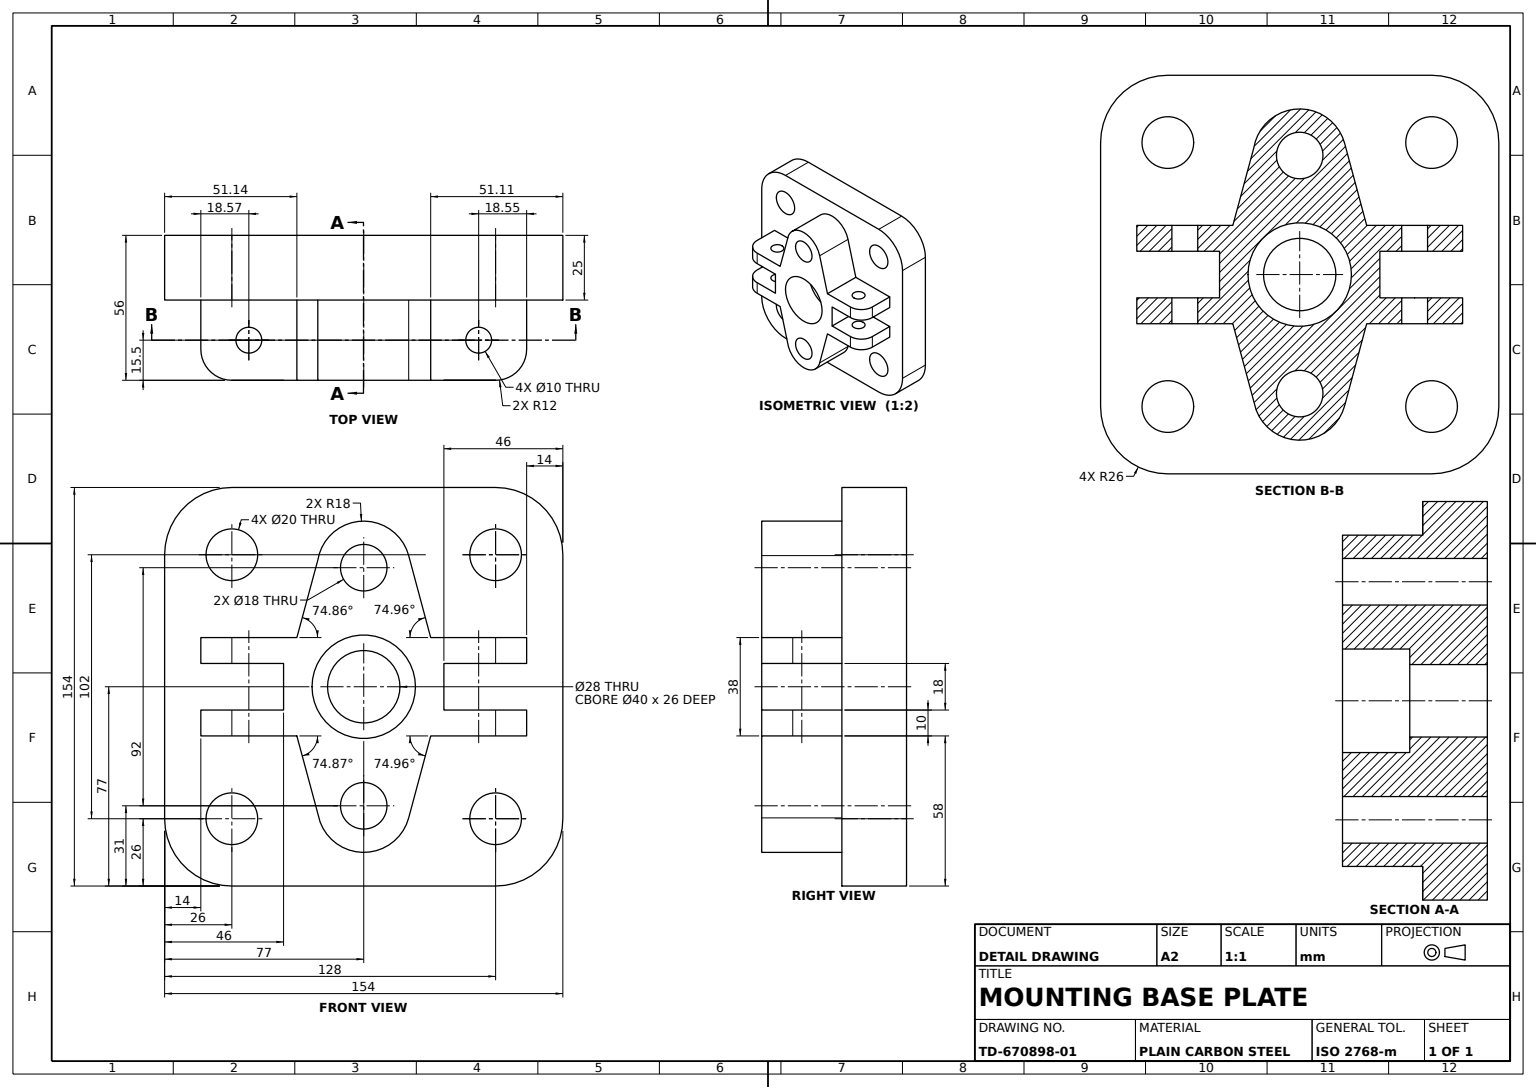
from build123d import *

# Parameters (mm, degrees)
BASE_PLATE_SKETCH_W        = 154
BASE_PLATE_SKETCH_H        = 154
BASE_PLATE_DEPTH           = 25
PLATE_CORNER_FILLETS_R26_R = 26
CORNER_HOLES_SKETCH_R      = 10
CORNER_HOLES_4X_20_DEPTH   = 25
CENTRAL_HUB_BOSS_DEPTH     = 31
CENTRE_TAP_DRILL_M20X2_0_D = 18
COUNTERBORE_SKETCH_R       = 14
COUNTERBORE_28_DEPTH       = 225.873297659
BORE_STEP_SKETCH_R         = 20
BORE_STEP_CUT_DEPTH        = 26
LUG_SLOT_A_SKETCH_R        = 5
LUG_SLOT_A_DEPTH           = 190.915770804
LUG_SLOT_B_SKETCH_R        = 5
LUG_SLOT_B_DEPTH           = 190.915770804
HUB_FILLETS_R12_R          = 12


with BuildPart() as part:
    # Base Plate Sketch → Base Plate (new body)
    with BuildSketch(Plane.XY):
        with Locations((77, 77)):
            Rectangle(BASE_PLATE_SKETCH_W, BASE_PLATE_SKETCH_H)
    extrude(amount=BASE_PLATE_DEPTH)

    # Plate Corner Fillets R26
    plate_corner_fillets_r26_edges = [part.edges().sort_by_distance(p)[0] for p in [
        (0, 154, 12.5),
        (154, 154, 12.5),
        (154, 0, 12.5),
        (0, 0, 12.5),
    ]]
    fillet(plate_corner_fillets_r26_edges, radius=PLATE_CORNER_FILLETS_R26_R)

    # Corner Holes Sketch → Corner Holes 4xØ20 (cut)
    with BuildSketch(Plane.XY.offset(25)):
        with Locations((26, 128)):
            Circle(CORNER_HOLES_SKETCH_R)
        with Locations((128, 128)):
            Circle(CORNER_HOLES_SKETCH_R)
        with Locations((128, 26)):
            Circle(CORNER_HOLES_SKETCH_R)
        with Locations((26, 26)):
            Circle(CORNER_HOLES_SKETCH_R)
    extrude(amount=-CORNER_HOLES_4X_20_DEPTH, mode=Mode.SUBTRACT)

    # Hub Profile Sketch → Central Hub Boss (add)
    with BuildSketch(Plane.XY.offset(25)):
        with BuildLine():
            Line((14, 58), (51.135796279, 58))
            Line((51.135796279, 58), (59.2634951, 27.931385667))
            Line((59.2634951, 27.931385667), (60.132879108, 24.715078934))
            ThreePointArc((60.132879108, 24.715078934), (77.84706214, 13.019941999), (94.383283675, 26.328656654))
            Line((94.383283675, 26.328656654), (102.894202658, 58))
            Line((102.894202658, 58), (140, 58))
            Line((140, 58), (140, 68))
            Line((140, 68), (108, 68))
            Line((108, 68), (108, 77))
            Line((108, 77), (108, 86))
            Line((108, 86), (140, 86))
            Line((140, 86), (140, 96))
            Line((140, 96), (102.894202658, 96))
            Line((102.894202658, 96), (94.383283675, 127.671343346))
            ThreePointArc((94.383283675, 127.671343346), (76.094284636, 140.977198883), (59.23523482, 125.900537557))
            Line((59.23523482, 125.900537557), (51.142468246, 96))
            Line((51.142468246, 96), (14, 96))
            Line((14, 96), (14, 86))
            Line((14, 86), (46, 86))
            Line((46, 86), (46, 77))
            Line((46, 77), (46, 68))
            Line((46, 68), (14, 68))
            Line((14, 68), (14, 58))
        make_face()
    extrude(amount=CENTRAL_HUB_BOSS_DEPTH)

    # Centre Tap Drill M20x2.0 (through all)
    with Locations(Plane.XY.offset(56)):
        with Locations((77, 123), (77, 31)):
            Hole(CENTRE_TAP_DRILL_M20X2_0_D / 2)

    # Counterbore Sketch → Counterbore Ø28 (cut, through all)
    with BuildSketch(Plane.XY.offset(56)):
        with Locations((77, 77)):
            Circle(COUNTERBORE_SKETCH_R)
    extrude(amount=-COUNTERBORE_28_DEPTH, mode=Mode.SUBTRACT)

    # Bore Step Sketch → Bore Step Cut (cut)
    with BuildSketch(Plane.XY.offset(56)):
        with Locations((77, 77)):
            Circle(BORE_STEP_SKETCH_R)
    extrude(amount=-BORE_STEP_CUT_DEPTH, mode=Mode.SUBTRACT)

    # Lug Slot A Sketch → Lug Slot A (cut, through all)
    with BuildSketch(Plane.XZ.offset(-58)):
        with Locations(Location((32.567898139, 40.5, 0), (0, 0, 270))):
            Circle(LUG_SLOT_A_SKETCH_R)
    extrude(amount=-LUG_SLOT_A_DEPTH, mode=Mode.SUBTRACT)

    # Lug Slot B Sketch → Lug Slot B (cut, through all)
    with BuildSketch(Plane.XZ.offset(-58)):
        with Locations((121.447101329, 40.5)):
            Circle(LUG_SLOT_B_SKETCH_R)
    extrude(amount=-LUG_SLOT_B_DEPTH, mode=Mode.SUBTRACT)

    # Hub Fillets R12
    hub_fillets_r12_edges = [part.edges().sort_by_distance(p)[0] for p in [
        (140, 63, 56),
        (14, 91, 56),
        (140, 91, 56),
        (14, 63, 56),
    ]]
    fillet(hub_fillets_r12_edges, radius=HUB_FILLETS_R12_R)


solid = part.part
